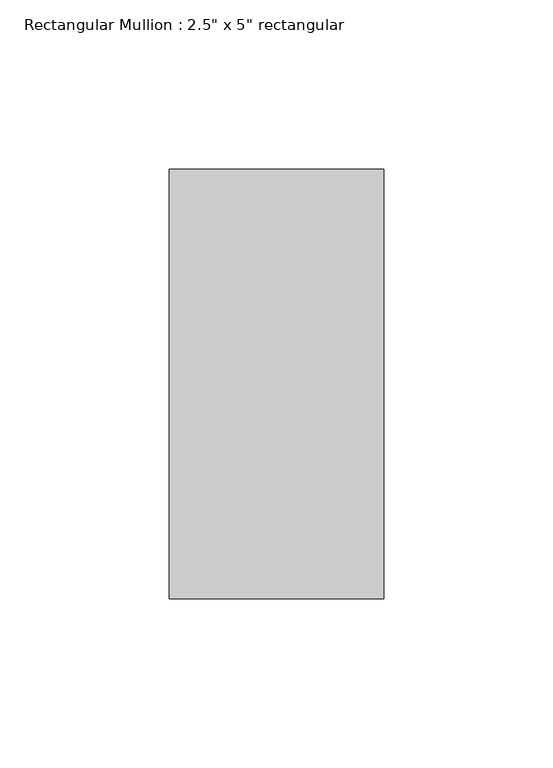
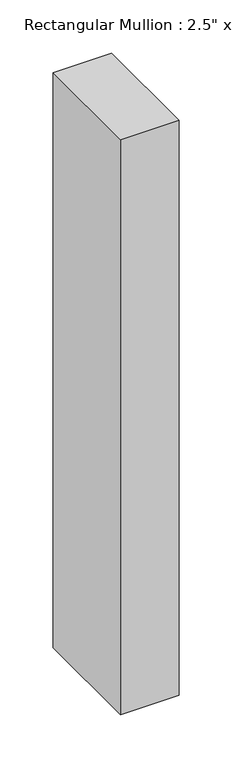
"""IFC4 building model written with IfcOpenShell, lengths in millimetres: member geometry."""

from ifc_helpers import new_model, si_unit, frame, origin, place, context, project, spatial, polyline, outline, extrude, source, transform, mapped, element, save


def member_a8964de5(model_context):
    return source(origin(), model_context, "Body", "SweptSolid", [
        extrude(outline(polyline([(0.0, 63.5), (0.0, -63.5), (-63.5, -63.5), (-63.5, 63.5), (0.0, 63.5)])), frame((0.0, 0.0, -660.5049172), z_axis=(0.0, 0.0, 1.0), x_axis=(1.0, 0.0, 0.0)), (0.0, 0.0, 1.0), 660.5049172),
    ])


if __name__ == "__main__":
    model = new_model("IFC4")
    model_context = context("Model", 3, world=origin())
    ifc_project = project(units=[si_unit("LENGTHUNIT", "METRE", prefix="MILLI")], contexts=[model_context])
    site = spatial("IfcSite", under=ifc_project)
    building = spatial("IfcBuilding", under=site)
    placement = place(None, origin())
    member_shape = member_a8964de5(model_context)
    element("IfcMember", 1, ObjectType="Rectangular Mullion : 2.5\" x 5\" rectangular", at=placement, inside=building, context=model_context, shape_type="MappedRepresentation", body=[
        mapped(member_shape, transform((0.0, 0.0, 0.0), x_axis=(1.0, 0.0, 0.0), y_axis=(0.0, 1.0, 0.0), z_axis=(0.0, 0.0, 1.0))),
    ])
    save(model, "model.ifc")

# Revit data of these elements
# Type "Rectangular Mullion : 2.5\" x 5\" rectangular"
#   built-in parameter 1007304 = 0.416667 (stored number, unit not read)
#   built-in parameter 1007301 = 0.104167 (stored number, unit not read)
#   built-in parameter 1007300 = 0.104167 (stored number, unit not read)
# Element 1 (IfcMember, "Rectangular Mullion : 2.5\" x 5\" rectangular")
#   Materials on its faces: "Aluminum"
# Materials
#   "Aluminum": class "Metal", colour RGB 247 247 247, transparency 0, Description = "Aluminum 6061", Cost = 0
